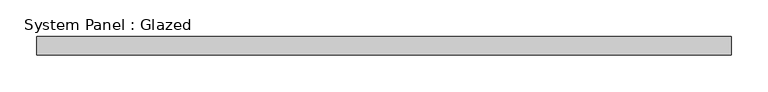
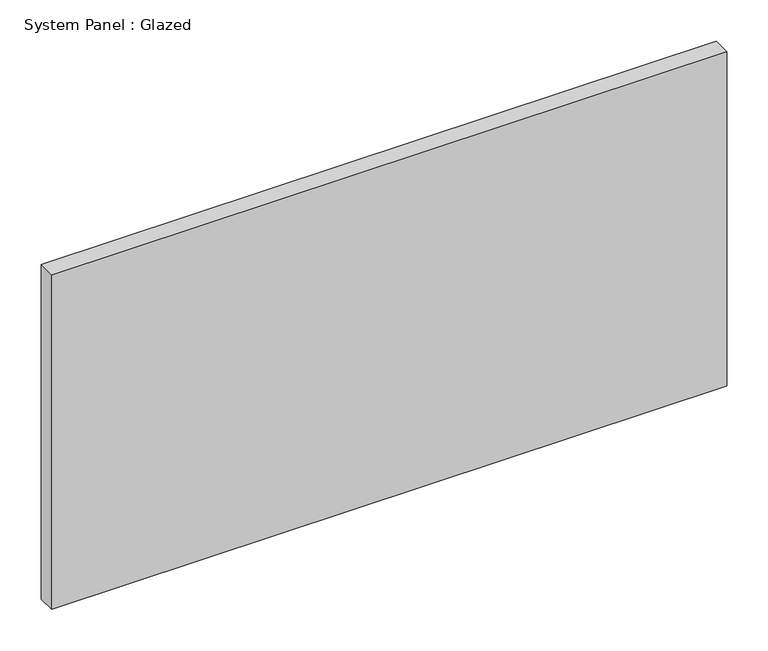
"""IFC4 building model written with IfcOpenShell, lengths in millimetres: plate geometry, System Panel : Glazed."""

from ifc_helpers import new_model, si_unit, origin, origin_with_axes, place, context, project, spatial, polyline, outline, extrude, source, transform, mapped, element, save


def system_panel_glazed_e3058915(model_context):
    return source(origin(), model_context, "Body", "SweptSolid", [
        extrude(outline(polyline([(472.28125, 19.05), (-472.28125, 19.05), (-472.28125, 44.45), (472.28125, 44.45), (472.28125, 19.05)])), origin_with_axes(), (0.0, 0.0, 1.0), 495.3),
    ])


if __name__ == "__main__":
    model = new_model("IFC4")
    model_context = context("Model", 3, world=origin())
    ifc_project = project(units=[si_unit("LENGTHUNIT", "METRE", prefix="MILLI")], contexts=[model_context])
    site = spatial("IfcSite", under=ifc_project)
    building = spatial("IfcBuilding", under=site)
    placement = place(None, origin())
    system_panel_glazed_shape = system_panel_glazed_e3058915(model_context)
    element("IfcPlate", 1, ObjectType="System Panel : Glazed", at=placement, inside=building, context=model_context, shape_type="MappedRepresentation", body=[
        mapped(system_panel_glazed_shape, transform((0.0, 0.0, 0.0), x_axis=(1.0, 0.0, 0.0), y_axis=(0.0, 1.0, 0.0), z_axis=(0.0, 0.0, 1.0))),
    ])
    save(model, "model.ifc")

# Revit data of these elements
# Type "System Panel : Glazed"
#   Construction Type Id = "GSP4R"
#   Analytic Construction = "1/8 in Pilkington single glazing"
#   Visual Light Transmittance = 0.9
#   Solar Heat Gain Coefficient = 0.86
#   Heat Transfer Coefficient (U) = 1.18115 BTU/(h·ft²·°F)
#   Define Thermal Properties by = 1
# Element 1 (IfcPlate, "System Panel : Glazed")
#   Materials on its faces: "Glass"
# Materials
#   "Glass": class "Glass", colour RGB 0 128 192, transparency 0.75, Description = "Soda Lime Glass", Cost = 0
